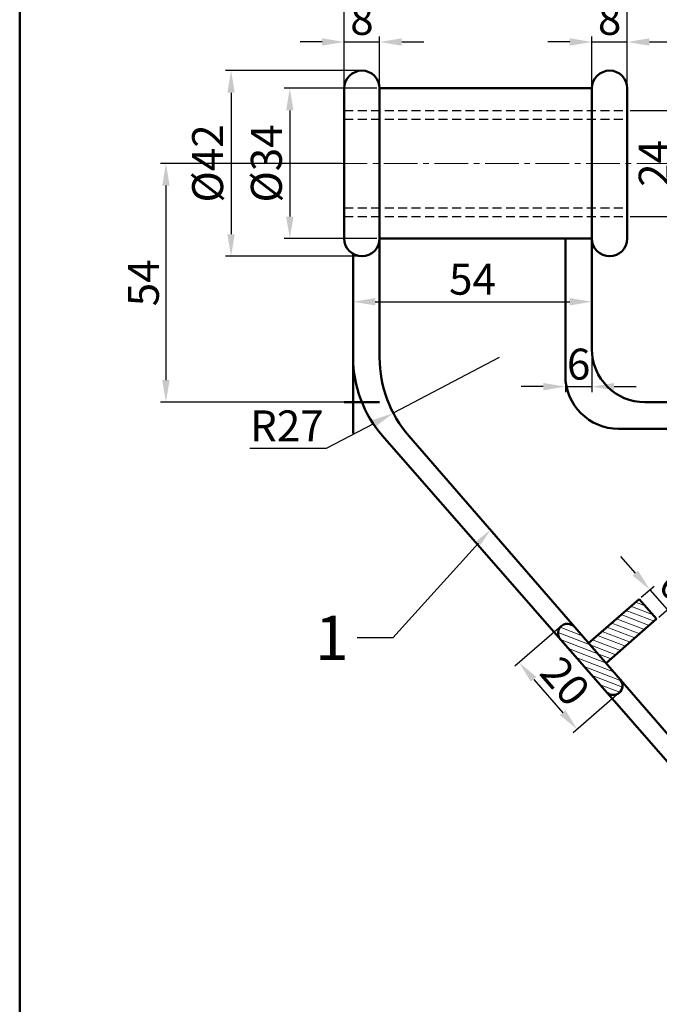
# Model space of a CAD drawing. Units: millimetres. Extents: x 434 to 1535, y -197 to 318.
# Tile 1 of 9: x 434 to 579, y -19 to 204. Entities that reach past the tile are written whole.
import ezdxf
from ezdxf import colors
from ezdxf.entities.mleader import LeaderData, LeaderLine
from ezdxf.math import Vec2, Vec3

# ---------------------------------------------------------------- set-up
doc = ezdxf.new("R2010")
doc.units = ezdxf.units.MM
doc.header["$LTSCALE"] = 0.4
doc.linetypes.add('CENTER2', pattern=[28.575, 19.05, -3.175, 3.175, -3.175])
doc.linetypes.add('DASHED', pattern=[19.05, 12.7, -6.35])
for name, color, linetype, lineweight in [('M-CNTR', 1, 'CENTER2', 18), ('M-DIMS', 2, 'Continuous', 25), ('M-HATC', 8, 'Continuous', 18), ('M-HIDN', 6, 'DASHED', 25), ('M-OUTL', 7, 'Continuous', 50), ('M-TEXT', 3, 'Continuous', 25)]:
    doc.layers.add(name, color=color, linetype=linetype, lineweight=lineweight)
doc.styles.get("Standard").update_dxf_attribs({"font": 'arial.ttf'})
doc.dimstyles.new('ISO-25', dxfattribs={"dimtxt": 7, "dimasz": 5, "dimexe": 1.25, "dimexo": 0.625, "dimtad": 1, "dimtoh": 1, "dimdec": 0, "dimtxsty": 'Standard', "dimcen": 2.5, "dimadec": 0, "dimazin": 0, "dimtfac": 1, "dimtdec": 0, "dimtmove": 0, "dimatfit": 3, "dimfxl": 1, "dimarcsym": 0})

# ---------------------------------------------------------------- blocks, each defined once
blk = doc.blocks.new('*U3')
at = {"layer": 'M-CNTR', "color": 0, "transparency": 16777216}
blk.add_line((-45.89, 0), (45.61, 0), dxfattribs=at)
blk = doc.blocks.new('*D7')
at = {"layer": 'Defpoints', "color": 0, "ltscale": 0.4, "transparency": 16777216}
for p in [(515.58, 199.04), (507.58, 188.56), (515.58, 188.56)]:
    blk.add_point(p, dxfattribs=at)
at = {"layer": 'M-DIMS', "color": 0, "lineweight": -2, "ltscale": 0.4, "transparency": 16777216}
for p, q in [((502.58, 199.04), (497.58, 199.04)), ((507.58, 189.19), (507.58, 200.29)), ((507.58, 199.04), (515.58, 199.04)), ((515.58, 189.19), (515.58, 200.29)), ((520.58, 199.04), (525.58, 199.04))]:
    blk.add_line(p, q, dxfattribs=at)
at = {"layer": 'M-DIMS', "color": 0, "ltscale": 0.4, "transparency": 16777216}
for points in [[(502.58, 199.87), (502.58, 198.21), (507.58, 199.04)], [(520.58, 199.87), (520.58, 198.21), (515.58, 199.04)]]:
    blk.add_solid(points, dxfattribs=at)
at = {"layer": 'M-DIMS', "color": 0, "ltscale": 0.4, "transparency": 16777216, "insert": (511.58, 203.24), "char_height": 7, "attachment_point": 5}
blk.add_mtext('8', dxfattribs=at)
blk = doc.blocks.new('*D8')
at = {"layer": 'Defpoints', "color": 0, "ltscale": 0.4, "transparency": 16777216}
for p in [(515.58, 188.56), (495.27, 154.56), (515.58, 154.56)]:
    blk.add_point(p, dxfattribs=at)
at = {"layer": 'M-DIMS', "color": 0, "lineweight": -2, "ltscale": 0.4, "transparency": 16777216}
for p, q in [((514.95, 188.56), (494.02, 188.56)), ((495.27, 183.56), (495.27, 159.56)), ((514.95, 154.56), (494.02, 154.56))]:
    blk.add_line(p, q, dxfattribs=at)
at = {"layer": 'M-DIMS', "color": 0, "ltscale": 0.4, "transparency": 16777216}
for points in [[(494.44, 183.56), (496.11, 183.56), (495.27, 188.56)], [(494.44, 159.56), (496.11, 159.56), (495.27, 154.56)]]:
    blk.add_solid(points, dxfattribs=at)
at = {"layer": 'M-DIMS', "color": 0, "ltscale": 0.4, "transparency": 16777216, "insert": (490.88, 171.56), "char_height": 7, "attachment_point": 5, "rotation": 90}
blk.add_mtext('%%C34', dxfattribs=at)
blk = doc.blocks.new('*D9')
at = {"layer": 'Defpoints', "color": 0, "ltscale": 0.4, "transparency": 16777216}
for p in [(511.58, 192.56), (481.99, 150.56), (511.58, 150.56)]:
    blk.add_point(p, dxfattribs=at)
at = {"layer": 'M-DIMS', "color": 0, "lineweight": -2, "ltscale": 0.4, "transparency": 16777216}
for p, q in [((510.95, 192.56), (480.74, 192.56)), ((481.99, 187.56), (481.99, 155.56)), ((510.95, 150.56), (480.74, 150.56))]:
    blk.add_line(p, q, dxfattribs=at)
at = {"layer": 'M-DIMS', "color": 0, "ltscale": 0.4, "transparency": 16777216}
for points in [[(481.16, 187.56), (482.82, 187.56), (481.99, 192.56)], [(481.16, 155.56), (482.82, 155.56), (481.99, 150.56)]]:
    blk.add_solid(points, dxfattribs=at)
at = {"layer": 'M-DIMS', "color": 0, "ltscale": 0.4, "transparency": 16777216, "insert": (477.6, 171.56), "char_height": 7, "attachment_point": 5, "rotation": 90}
blk.add_mtext('%%C42', dxfattribs=at)
blk = doc.blocks.new('*D10')
at = {"layer": 'Defpoints', "color": 0, "ltscale": 0.4, "transparency": 16777216}
for p in [(507.58, 171.56), (467.26, 117.56), (509.58, 117.56)]:
    blk.add_point(p, dxfattribs=at)
at = {"layer": 'M-DIMS', "color": 0, "lineweight": -2, "ltscale": 0.4, "transparency": 16777216}
for p, q in [((506.95, 171.56), (466.01, 171.56)), ((467.26, 166.56), (467.26, 122.56)), ((508.95, 117.56), (466.01, 117.56))]:
    blk.add_line(p, q, dxfattribs=at)
at = {"layer": 'M-DIMS', "color": 0, "ltscale": 0.4, "transparency": 16777216}
for points in [[(466.43, 166.56), (468.09, 166.56), (467.26, 171.56)], [(466.43, 122.56), (468.09, 122.56), (467.26, 117.56)]]:
    blk.add_solid(points, dxfattribs=at)
at = {"layer": 'M-DIMS', "color": 0, "ltscale": 0.4, "transparency": 16777216, "insert": (463.07, 144.56), "char_height": 7, "attachment_point": 5, "rotation": 90}
blk.add_mtext('54', dxfattribs=at)
blk = doc.blocks.new('*D11')
at = {"layer": 'Defpoints', "color": 0, "ltscale": 0.4, "transparency": 16777216}
for p in [(571.58, 213.45), (507.58, 188.56), (571.58, 185.87)]:
    blk.add_point(p, dxfattribs=at)
at = {"layer": 'M-DIMS', "color": 0, "lineweight": -2, "ltscale": 0.4, "transparency": 16777216}
for p, q in [((507.58, 189.19), (507.58, 214.7)), ((571.58, 186.49), (571.58, 214.7)), ((512.58, 213.45), (566.58, 213.45))]:
    blk.add_line(p, q, dxfattribs=at)
at = {"layer": 'M-DIMS', "color": 0, "ltscale": 0.4, "transparency": 16777216}
for points in [[(512.58, 214.29), (512.58, 212.62), (507.58, 213.45)], [(566.58, 214.29), (566.58, 212.62), (571.58, 213.45)]]:
    blk.add_solid(points, dxfattribs=at)
at = {"layer": 'M-DIMS', "color": 0, "ltscale": 0.4, "transparency": 16777216, "insert": (539.58, 217.65), "char_height": 7, "attachment_point": 5}
blk.add_mtext('64', dxfattribs=at)
blk = doc.blocks.new('*D12')
at = {"layer": 'Defpoints', "color": 0, "ltscale": 0.4, "transparency": 16777216}
for p in [(571.58, 199.04), (563.58, 188.56), (571.58, 188.56)]:
    blk.add_point(p, dxfattribs=at)
at = {"layer": 'M-DIMS', "color": 0, "lineweight": -2, "ltscale": 0.4, "transparency": 16777216}
for p, q in [((558.58, 199.04), (553.58, 199.04)), ((563.58, 189.19), (563.58, 200.29)), ((563.58, 199.04), (571.58, 199.04)), ((571.58, 189.19), (571.58, 200.29)), ((576.58, 199.04), (581.58, 199.04))]:
    blk.add_line(p, q, dxfattribs=at)
at = {"layer": 'M-DIMS', "color": 0, "ltscale": 0.4, "transparency": 16777216}
for points in [[(558.58, 199.87), (558.58, 198.21), (563.58, 199.04)], [(576.58, 199.87), (576.58, 198.21), (571.58, 199.04)]]:
    blk.add_solid(points, dxfattribs=at)
at = {"layer": 'M-DIMS', "color": 0, "ltscale": 0.4, "transparency": 16777216, "insert": (567.58, 203.24), "char_height": 7, "attachment_point": 5}
blk.add_mtext('8', dxfattribs=at)
blk = doc.blocks.new('*D13')
at = {"layer": 'Defpoints', "color": 0, "ltscale": 0.4, "transparency": 16777216}
for p in [(571.58, 183.56), (571.58, 159.56), (582.71, 159.56)]:
    blk.add_point(p, dxfattribs=at)
at = {"layer": 'M-DIMS', "color": 0, "lineweight": -2, "ltscale": 0.4, "transparency": 16777216}
for p, q in [((572.2, 183.56), (583.96, 183.56)), ((582.71, 178.56), (582.71, 164.56)), ((572.2, 159.56), (583.96, 159.56))]:
    blk.add_line(p, q, dxfattribs=at)
at = {"layer": 'M-DIMS', "color": 0, "ltscale": 0.4, "transparency": 16777216}
for points in [[(581.87, 178.56), (583.54, 178.56), (582.71, 183.56)], [(581.87, 164.56), (583.54, 164.56), (582.71, 159.56)]]:
    blk.add_solid(points, dxfattribs=at)
at = {"layer": 'M-DIMS', "color": 0, "ltscale": 0.4, "transparency": 16777216, "insert": (578.57, 171.56), "char_height": 7, "attachment_point": 5, "rotation": 90}
blk.add_mtext('24', dxfattribs=at)
blk = doc.blocks.new('*D14')
at = {"layer": 'Defpoints', "color": 0, "ltscale": 0.4, "transparency": 16777216}
for p in [(509.58, 141.14), (563.58, 141.14), (563.58, 140.29)]:
    blk.add_point(p, dxfattribs=at)
at = {"layer": 'M-DIMS', "color": 0, "lineweight": -2, "ltscale": 0.4, "transparency": 16777216}
for p, q in [((509.58, 140.51), (509.58, 139.04)), ((563.58, 140.51), (563.58, 139.04)), ((514.58, 140.29), (558.58, 140.29))]:
    blk.add_line(p, q, dxfattribs=at)
at = {"layer": 'M-DIMS', "color": 0, "ltscale": 0.4, "transparency": 16777216}
for points in [[(514.58, 141.12), (514.58, 139.45), (509.58, 140.29)], [(558.58, 141.12), (558.58, 139.45), (563.58, 140.29)]]:
    blk.add_solid(points, dxfattribs=at)
at = {"layer": 'M-DIMS', "color": 0, "ltscale": 0.4, "transparency": 16777216, "insert": (536.58, 144.47), "char_height": 7, "attachment_point": 5}
blk.add_mtext('54', dxfattribs=at)
blk = doc.blocks.new('*D15')
at = {"layer": 'Defpoints', "color": 0, "ltscale": 0.4, "transparency": 16777216}
for p in [(557.58, 132.22), (563.58, 132.22), (563.58, 121.08)]:
    blk.add_point(p, dxfattribs=at)
at = {"layer": 'M-DIMS', "color": 0, "lineweight": -2, "ltscale": 0.4, "transparency": 16777216}
for p, q in [((557.58, 131.59), (557.58, 119.83)), ((563.58, 131.59), (563.58, 119.83)), ((552.58, 121.08), (547.58, 121.08)), ((557.58, 121.08), (563.58, 121.08)), ((568.58, 121.08), (573.58, 121.08))]:
    blk.add_line(p, q, dxfattribs=at)
at = {"layer": 'M-DIMS', "color": 0, "ltscale": 0.4, "transparency": 16777216}
for points in [[(552.58, 121.91), (552.58, 120.24), (557.58, 121.08)], [(568.58, 121.91), (568.58, 120.24), (563.58, 121.08)]]:
    blk.add_solid(points, dxfattribs=at)
at = {"layer": 'M-DIMS', "color": 0, "ltscale": 0.4, "transparency": 16777216, "insert": (560.58, 125.27), "char_height": 7, "attachment_point": 5}
blk.add_mtext('6', dxfattribs=at)
blk = doc.blocks.new('*D20')
at = {"layer": 'Defpoints', "color": 0, "ltscale": 0.4, "transparency": 16777216}
for p in [(556.65, 66.94), (569.78, 51.86), (560.26, 43.57)]:
    blk.add_point(p, dxfattribs=at)
at = {"layer": 'M-DIMS', "color": 0, "lineweight": -2, "ltscale": 0.4, "transparency": 16777216}
for p, q in [((556.18, 66.53), (546.18, 57.83)), ((550.41, 54.88), (556.98, 47.34)), ((569.31, 51.45), (559.32, 42.75))]:
    blk.add_line(p, q, dxfattribs=at)
at = {"layer": 'M-DIMS', "color": 0, "ltscale": 0.4, "transparency": 16777216}
for points in [[(551.04, 55.43), (549.78, 54.33), (547.13, 58.65)], [(557.61, 47.88), (556.35, 46.79), (560.26, 43.57)]]:
    blk.add_solid(points, dxfattribs=at)
at = {"layer": 'M-DIMS', "color": 0, "ltscale": 0.4, "transparency": 16777216, "insert": (556.86, 53.87), "char_height": 7, "attachment_point": 5, "rotation": 311.0428}
blk.add_mtext('20', dxfattribs=at)
blk = doc.blocks.new('*D21')
at = {"layer": 'Defpoints', "color": 0, "ltscale": 0.4, "transparency": 16777216}
for p in [(574.27, 73.05), (580.63, 70.64), (578.22, 68.53)]:
    blk.add_point(p, dxfattribs=at)
at = {"layer": 'M-DIMS', "color": 0, "lineweight": -2, "ltscale": 0.4, "transparency": 16777216}
for p, q in [((573.4, 78.92), (570.11, 82.68)), ((574.74, 73.46), (577.63, 75.98)), ((576.69, 75.15), (580.63, 70.64)), ((578.69, 68.94), (581.58, 71.46)), ((583.92, 66.87), (587.21, 63.11))]:
    blk.add_line(p, q, dxfattribs=at)
at = {"layer": 'M-DIMS', "color": 0, "ltscale": 0.4, "transparency": 16777216}
for points in [[(574.02, 79.47), (572.77, 78.37), (576.69, 75.15)], [(584.55, 67.42), (583.3, 66.32), (580.63, 70.64)]]:
    blk.add_solid(points, dxfattribs=at)
at = {"layer": 'M-DIMS', "color": 0, "ltscale": 0.4, "transparency": 16777216, "insert": (581.82, 75.66), "char_height": 7, "attachment_point": 5, "rotation": 311.1518}
blk.add_mtext('6', dxfattribs=at)
blk = doc.blocks.new('*D43')
at = {"layer": 'Defpoints', "color": 0, "ltscale": 0.4, "transparency": 16777216}
for p in [(542.58, 127.64), (518.67, 115.08)]:
    blk.add_point(p, dxfattribs=at)
at = {"layer": 'M-DIMS', "color": 0, "lineweight": -2, "ltscale": 0.4, "transparency": 16777216}
for p, q in [((542.58, 127.64), (518.67, 115.08)), ((503.6, 107.16), (514.25, 112.75)), ((486.25, 107.16), (503.6, 107.16))]:
    blk.add_line(p, q, dxfattribs=at)
at = {"layer": 'M-DIMS', "color": 0, "ltscale": 0.4, "transparency": 16777216}
blk.add_solid([(513.86, 113.49), (514.64, 112.01), (518.67, 115.08)], dxfattribs=at)
at = {"layer": 'M-DIMS', "color": 0, "ltscale": 0.4, "transparency": 16777216, "insert": (494.61, 111.3), "char_height": 7, "attachment_point": 5}
blk.add_mtext('R27', dxfattribs=at)

msp = doc.modelspace()

# ---------------------------------------------------------------- hatches: boundary and pattern name
at = {"layer": 'M-HATC', "ltscale": 0.4}
h = msp.add_hatch(dxfattribs=at)
h.set_pattern_fill('ANSI31', color=256, scale=0.4, angle=114)
h.paths.add_polyline_path([(578.22, 68.53), (574.27, 73.05), (562.84, 63.06), (566.77, 58.52)])
h.paths.add_polyline_path([(559.66, 66.73, 1.001905), (556.44, 63.93), (566.82, 52.06, 0.998098), (569.99, 54.82)])

# ---------------------------------------------------------------- linework, layer by layer
at = {"layer": 'M-HIDN', "ltscale": 0.4}
for p, q in [((507.58, 183.56), (571.58, 183.56)), ((507.58, 181.56), (571.58, 181.56)), ((507.58, 161.56), (571.58, 161.56)), ((507.58, 159.56), (571.58, 159.56))]:
    msp.add_line(p, q, dxfattribs=at)
at = {"layer": 'M-OUTL', "ltscale": 0.4}
for p, q in [((507.58, 154.56), (507.58, 188.56)), ((515.58, 188.56), (515.58, 154.56)), ((515.58, 188.56), (563.58, 188.56)), ((563.58, 154.56), (563.58, 188.56)), ((571.58, 188.56), (571.58, 154.56)), ((515.58, 154.56), (563.58, 154.56)), ((515.58, 127.64), (515.58, 154.56)), ((557.58, 154.56), (557.58, 123.56)), ((563.58, 154.56), (563.58, 129.56)), ((509.58, 110.5), (509.58, 151.1)), ((507.58, 117.56), (515.58, 117.56)), ((647.58, 117.56), (575.58, 117.56)), ((647.58, 111.56), (569.58, 111.56)), ((516.24, 109.93), (607, 6.08)), ((607, 12.15), (522.18, 109.95)), ((562.84, 63.06), (574.27, 73.05)), ((574.27, 73.05), (578.22, 68.53)), ((566.77, 58.52), (578.22, 68.53))]:
    msp.add_line(p, q, dxfattribs=at)
msp.add_lwpolyline([(434.2, 318.45), (1535.47, 318.45), (1535.47, -197.48), (434.2, -197.48)], close=True, dxfattribs=at)
for centre, radius, start, end in [((511.58, 188.56), 4, 0, 180), ((567.58, 188.56), 4, 0, 180), ((511.58, 154.56), 4, 180, 0), ((567.58, 154.56), 4, 180, 0), ((575.58, 129.56), 12, 180, 270), ((536.58, 127.7), 27, 180, 221.1518), ((542.58, 127.64), 27, 180, 220.9337), ((569.58, 123.56), 12, 180, 270), ((558.05, 65.33), 2.13, 40.9337, 221.1518), ((568.4, 53.44), 2.1, 221.1518, 40.9337)]:
    msp.add_arc(centre, radius, start, end, dxfattribs=at)

# ---------------------------------------------------------------- block references
at = {"layer": 'M-CNTR'}
msp.add_blockref('*U3', (539.58, 171.56), dxfattribs=at)

# ---------------------------------------------------------------- dimensions: what is measured, and where the dimension line sits
at = {"layer": 'M-DIMS', "ltscale": 0.4}
for base, p1, p2, picture, middle in [((571.58, 213.45), (507.58, 188.56), (571.58, 185.87), '*D11', (539.58, 217.65)), ((515.58, 199.04), (507.58, 188.56), (515.58, 188.56), '*D7', (511.58, 203.24)), ((571.58, 199.04), (563.58, 188.56), (571.58, 188.56), '*D12', (567.58, 203.24)), ((563.58, 140.29), (509.58, 141.14), (563.58, 141.14), '*D14', (536.58, 144.47)), ((563.58, 121.08), (557.58, 132.22), (563.58, 132.22), '*D15', (560.58, 125.27))]:
    dim = msp.add_linear_dim(base=base, p1=p1, p2=p2, dimstyle='ISO-25', override={"dimclrd": 0, "dimclre": 0, "dimclrt": 0}, dxfattribs=at)
    dim.commit()
    dim.dimension.update_dxf_attribs({"geometry": picture, "text_midpoint": middle})
for base, p1, p2, picture, middle in [((481.99, 150.56), (511.58, 192.56), (511.58, 150.56), '*D9', (477.6, 171.56)), ((495.27, 154.56), (515.58, 188.56), (515.58, 154.56), '*D8', (490.88, 171.56))]:
    dim = msp.add_linear_dim(base=base, p1=p1, p2=p2, angle=90, text='%%C<>', dimstyle='ISO-25', override={"dimclrd": 0, "dimclre": 0, "dimclrt": 0}, dxfattribs=at)
    dim.commit()
    dim.dimension.update_dxf_attribs({"geometry": picture, "text_midpoint": middle})
for base, p1, p2, picture, middle in [((582.71, 159.56), (571.58, 183.56), (571.58, 159.56), '*D13', (578.57, 171.56)), ((467.26, 117.56), (507.58, 171.56), (509.58, 117.56), '*D10', (463.07, 144.56))]:
    dim = msp.add_linear_dim(base=base, p1=p1, p2=p2, angle=90, dimstyle='ISO-25', override={"dimclrd": 0, "dimclre": 0, "dimclrt": 0}, dxfattribs=at)
    dim.commit()
    dim.dimension.update_dxf_attribs({"geometry": picture, "text_midpoint": middle})
dim = msp.add_radius_dim(center=(542.58, 127.64), mpoint=(518.67, 115.08), dimstyle='ISO-25', override={"dimclrd": 0, "dimclre": 0, "dimclrt": 0}, dxfattribs=at)
dim.commit()
dim.dimension.update_dxf_attribs({"geometry": '*D43', "text_midpoint": (494.61, 111.3)})
for p1, p2, distance, picture, middle in [((574.27, 73.05), (578.22, 68.53), 3.2, '*D21', (581.82, 75.66)), ((556.65, 66.94), (569.78, 51.86), -12.63, '*D20', (556.86, 53.87))]:
    dim = msp.add_aligned_dim(p1=p1, p2=p2, distance=distance, dimstyle='ISO-25', override={"dimclrd": 0, "dimclre": 0, "dimclrt": 0}, dxfattribs=at)
    dim.commit()
    dim.dimension.update_dxf_attribs({"geometry": picture, "text_midpoint": middle})

# ---------------------------------------------------------------- leaders
at = {"layer": 'M-TEXT', "ltscale": 0.4}
ml = msp.add_multileader_mtext('Standard', dxfattribs=at)
ml.set_content('1', color=256)
ml.set_leader_properties()
ml.build(insert=Vec2(0, 0))
ctx = ml.context
ctx.base_point, ctx.char_height, ctx.plane_origin = Vec3(502.84, 64.26), 10, Vec3(540.62, 88.68)
ctx.text_align_type = 2
notes = []
notes.append((ctx, [(0, (1, 1, 0), (518.53, 64.26), (-1, 0), 8, [(0, [(540.62, 88.68)], 0, [])])]))
ctx.mtext.insert, ctx.mtext.alignment, ctx.mtext.flow_direction = Vec3(508.53, 69.26), 3, 5
for ctx, leaders in notes:
    for number, flags, end, landing, length, lines in leaders:
        leader = LeaderData()
        leader.index, (leader.has_last_leader_line, leader.has_dogleg_vector, leader.attachment_direction) = number, flags
        leader.last_leader_point, leader.dogleg_vector, leader.dogleg_length = Vec3(end), Vec3(landing), length
        for number, points, colour, breaks in lines:
            line = LeaderLine()
            line.index, line.vertices, line.color, line.breaks = number, Vec3.list(points), colors.encode_raw_color(colour), breaks
            leader.lines.append(line)
        ctx.leaders.append(leader)

doc.saveas('drawing.dxf')
